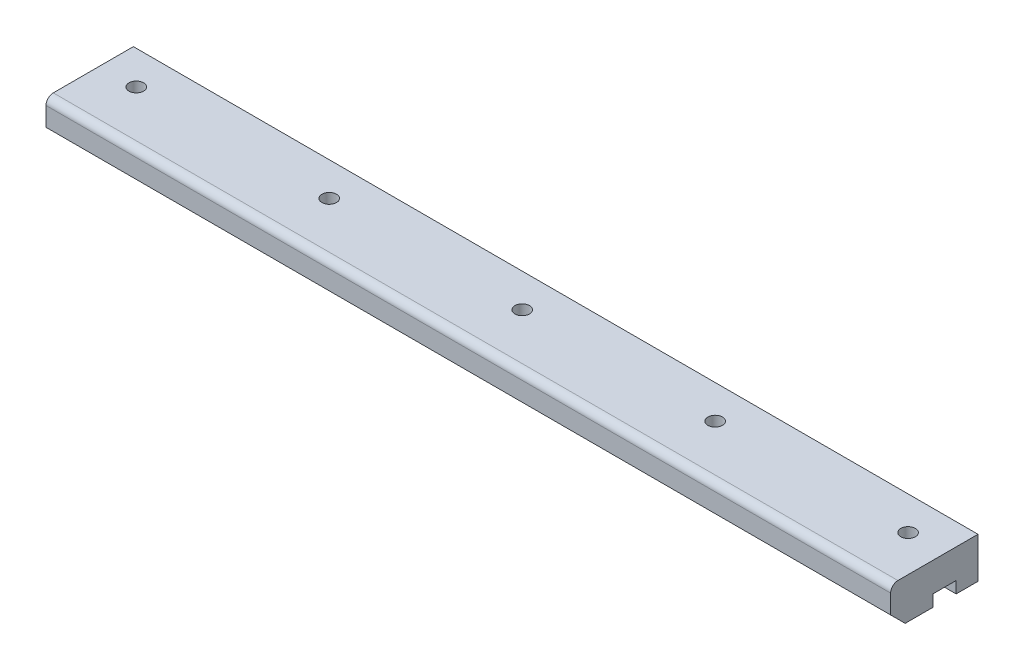
from build123d import *

# Parameters (mm, degrees)
RAIL_BODY_580_DEPTH        = 580
MOUNTING_HOLES_SKETCH_R    = 5
MOUNTING_HOLES_5X_10_DEPTH = 580


with BuildPart() as part:
    # Rail Profile Sketch → Rail Body 580 (new body)
    with BuildSketch(Plane(origin=(0, 0, 0), x_dir=(0, 0, -1), z_dir=(1, 0, 0))):
        with BuildLine():
            Line((-30, 10), (-30, 23))
            ThreePointArc((-30, 23), (-28.535533906, 26.535533906), (-25, 28))
            Line((-25, 28), (30, 28))
            Line((30, 28), (30, 0))
            Line((30, 0), (15, 0))
            Line((15, 0), (15, 8))
            Line((15, 8), (-1, 8))
            Line((-1, 8), (-1, 0))
            Line((-1, 0), (-20, 0))
            Line((-20, 0), (-30, 10))
        make_face()
    extrude(amount=RAIL_BODY_580_DEPTH)

    # Mounting Holes Sketch → Mounting Holes 5xØ10 (cut)
    with BuildSketch(Plane(origin=(0, 28, 0), x_dir=(1, 0, 0), z_dir=(0, 1, 0))):
        with Locations(Location((25, 7, 0), (0, 0, 270))):
            Circle(MOUNTING_HOLES_SKETCH_R)
        with Locations(Location((157.5, 7, 0), (0, 0, 270))):
            Circle(MOUNTING_HOLES_SKETCH_R)
        with Locations(Location((290, 7, 0), (0, 0, 270))):
            Circle(MOUNTING_HOLES_SKETCH_R)
        with Locations(Location((422.5, 7, 0), (0, 0, 270))):
            Circle(MOUNTING_HOLES_SKETCH_R)
        with Locations(Location((555, 7, 0), (0, 0, 270))):
            Circle(MOUNTING_HOLES_SKETCH_R)
    extrude(amount=-MOUNTING_HOLES_5X_10_DEPTH, mode=Mode.SUBTRACT)


solid = part.part
